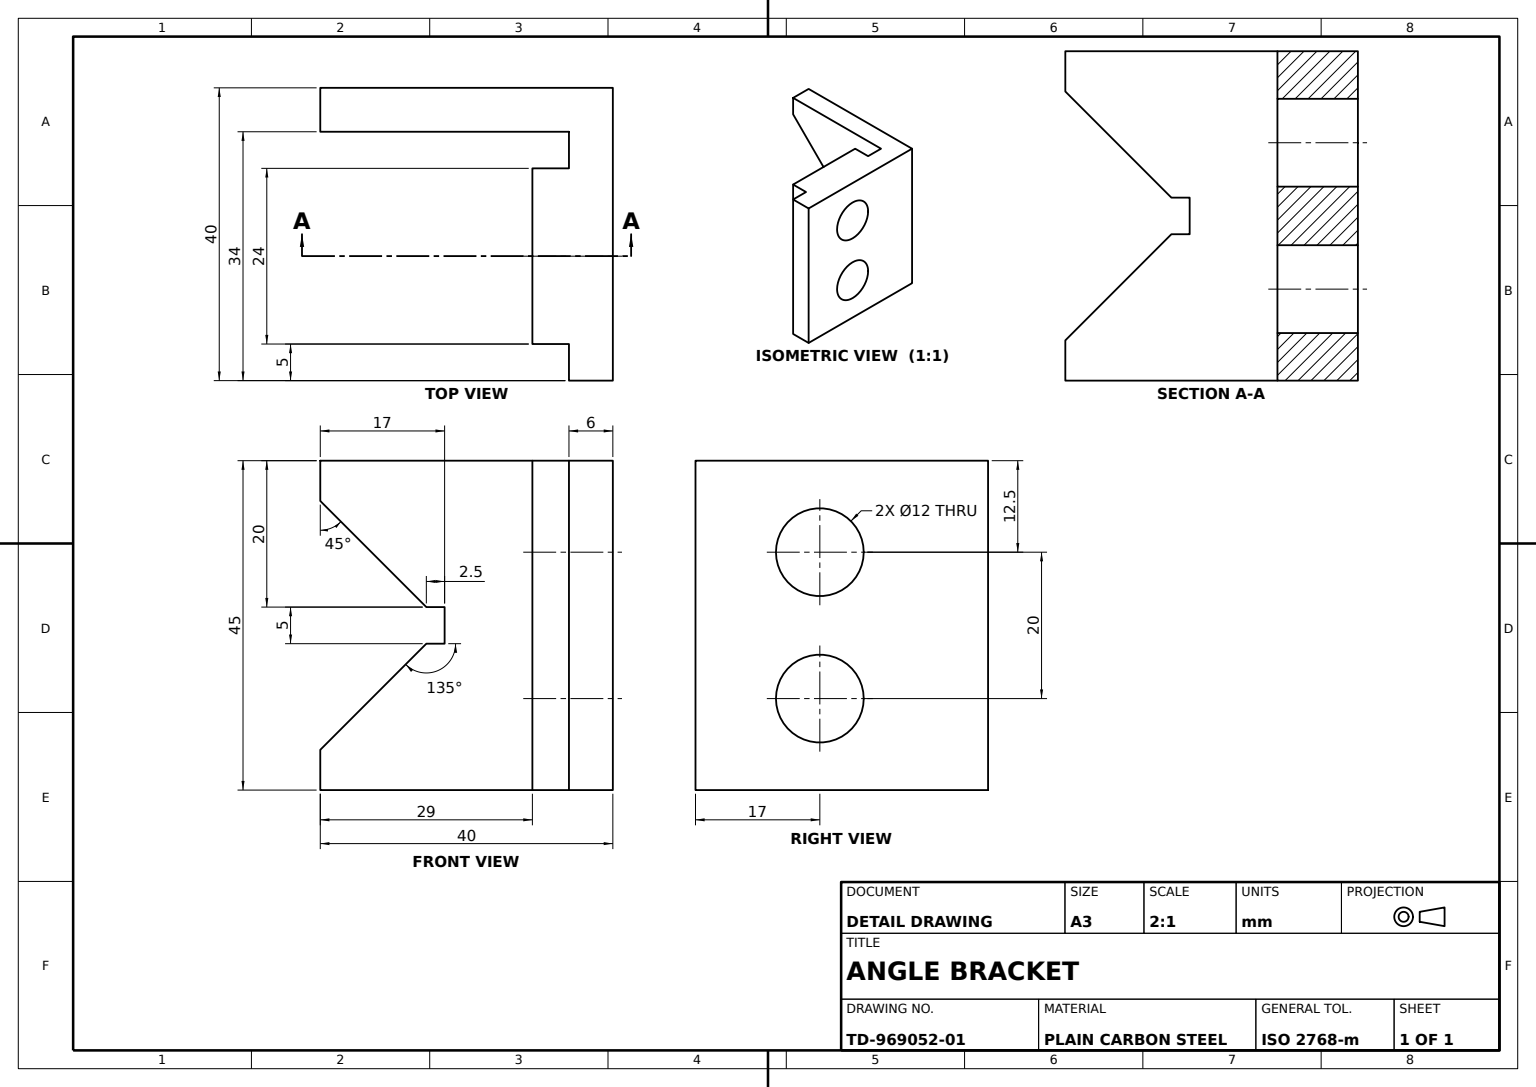
SolidWorks part; units mm, degrees
material "Plain Carbon Steel"
ref_plane "Front Plane" through (0, 0, 0) normal (0, 0, 1) x (1, 0, 0)
ref_plane "Top Plane" through (0, 0, 0) normal (0, 1, 0) x (1, 0, 0)
ref_plane "Right Plane" through (0, 0, 0) normal (1, 0, 0) x (0, 0, -1)
sketch "Base Plate Sketch" plane through (0, 0, 0) normal (0, 0, 1) x (1, 0, 0)
  line L0 (0, 0) -> (40, 0)
  line L1 (40, 0) -> (40, 45)
  line L2 (40, 45) -> (0, 45)
  line L3 (0, 45) -> (0, 0)
  dimension "D1" = 40
  dimension "D2" = 45
  dimension "D3" = 40
extrude "Base Plate" add sketch "Base Plate Sketch" along normal blind 6
sketch "Upright Flange Sketch" plane through (40, 0, 0) normal (1, 0, 0) x (0, 0, -1)
  line L0 (-6, 45) -> (-40, 45)
  line L1 (-40, 45) -> (-40, 0)
  line L2 (-40, 0) -> (-6, 0)
  line L3 (-6, 0) -> (-6, 45)
  dimension "D1" = 34
  dimension "D2" = 45
  dimension "D3" = 34
extrude "Upright Flange" add sketch "Upright Flange Sketch" against normal blind 6
sketch "Support Web Sketch" plane through (0, 0, 0) normal (0, -1, 0) x (1, 0, 0)
  line L0 (0, 6) -> (34, 6) construction
  line L1 (34, 40) -> (34, 6) construction
  line L2 (34, 35) -> (29, 35)
  line L3 (29, 35) -> (29, 11)
  line L4 (29, 11) -> (34, 11)
  line L5 (34, 11) -> (34, 35)
  dimension "D1" = 29
  dimension "D2" = 5
  dimension "D3" = 24
extrude "Support Web" add sketch "Support Web Sketch" against normal blind 45
sketch "Corner Relief Groove Sketch" plane through (0, 0, 6) normal (0, 0, 1) x (1, 0, 0)
  line L0 (0, 22.5) -> (17, 22.5)
  line L1 (0, 45) -> (0, 0) construction
  line L2 (17, 22.5) -> (17, 25)
  line L3 (17, 22.5) -> (17, 20)
  line L4 (17, 25) -> (14.5, 25)
  line L5 (17, 20) -> (14.5, 20)
  line L6 (0, 22.5) -> (0, 39.5)
  line L7 (0, 39.5) -> (0, 5.5)
  line L8 (0, 22.5) -> (0, 5.5)
  line L9 (0, 5.5) -> (14.5, 20)
  line L10 (0, 39.5) -> (14.5, 25)
  line M7 (0, 45) -> (0, 0)
  dimension "D1" = 17
  dimension "D2" = 2.5
  dimension "D3" = 2.5
  dimension "D4" = 2.5
  dimension "D5" = 2.5
  dimension "D6" = 45
  dimension "D7" = 45
extrude "Corner Relief Groove" cut sketch "Corner Relief Groove Sketch" against normal blind 45 contours L10 L0 L2 L4 M7 | L9 L5 L3 L0 M7
sketch "Mounting Holes Sketch" plane through (29, 0, 0) normal (-1, 0, 0) x (0, 0, 1)
  line L0 (35, 45) -> (35, 0) construction
  line L1 (35, 45) -> (35, 0) construction
  line L2 (35, 0) -> (11, 0) construction
  line L3 (35, 45) -> (11, 45) construction
  circle A0 centre (23, 32.5) radius 6
  circle A1 centre (23, 12.5) radius 6
  dimension "D1" = 6
  dimension "D2" = 6
  dimension "D3" = 12
  dimension "D4" = 12
  dimension "D5" = 12.5
  dimension "D6" = 12.5
extrude "Mounting Holes 2x" cut sketch "Mounting Holes Sketch" against normal blind 45
